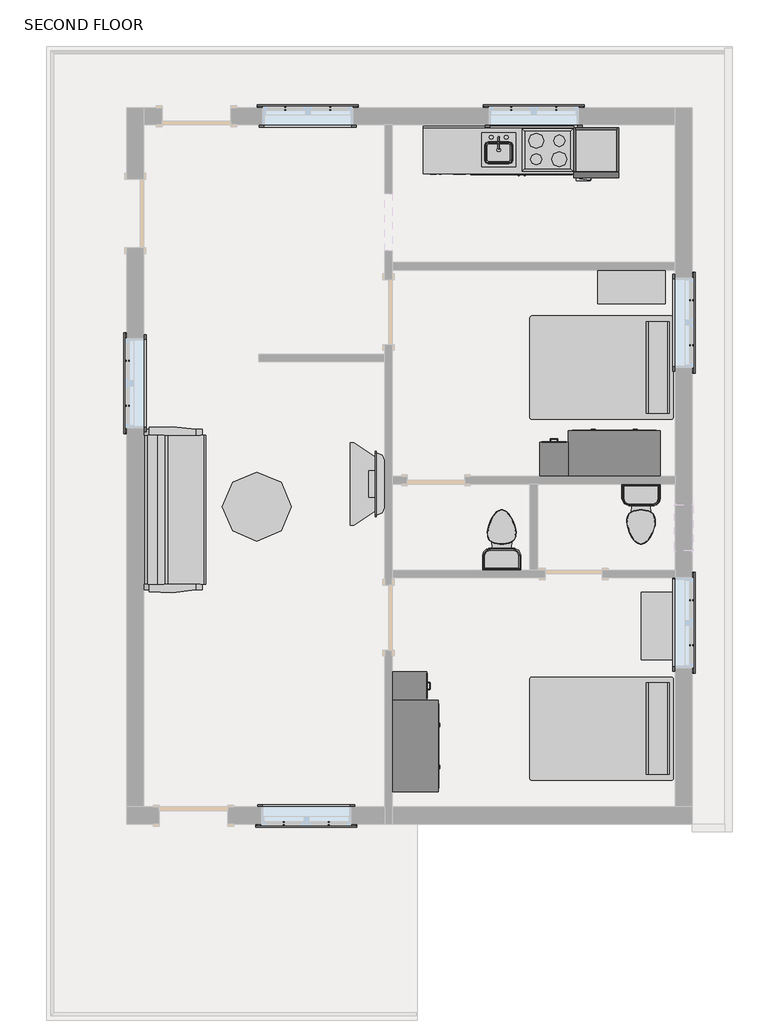
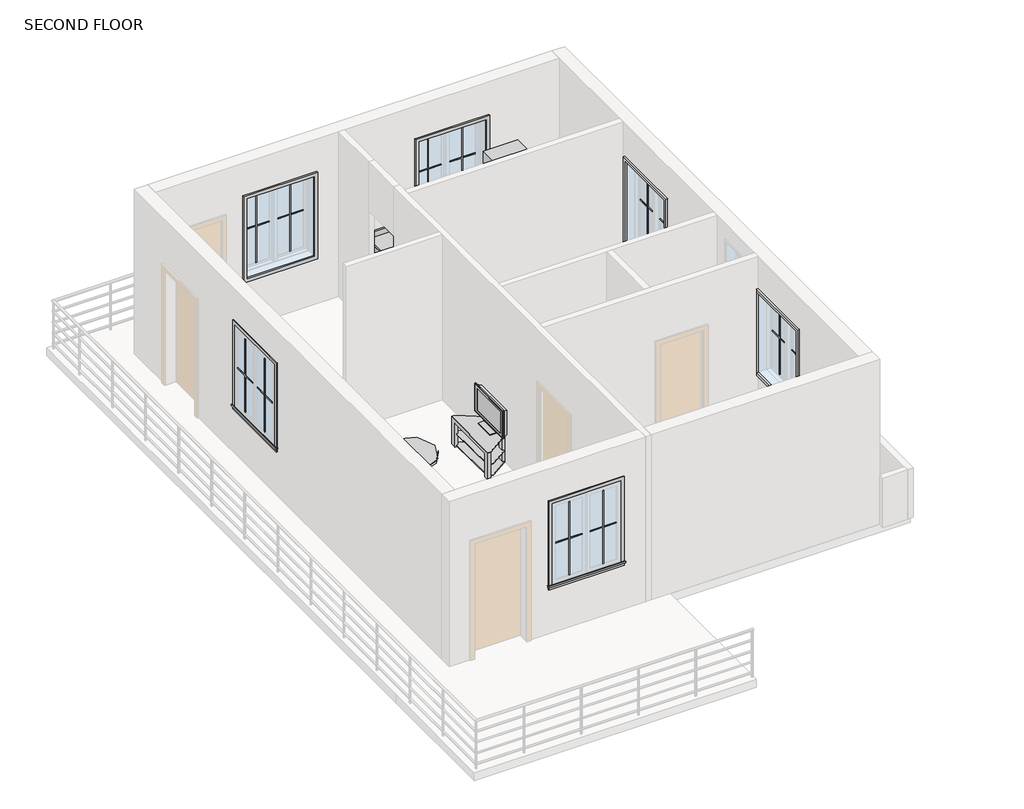
# One storey, part 3 of 3: 28 proxies, 13 furniture elements, 3 flow terminals.
"""IFC4 building model written with IfcOpenShell, lengths in millimetres."""

from ifc_helpers import new_model, si_unit, origin, place, context, project, spatial, transform, mapped, element, save
from components import m_cook_top_4_unit2_0615_x_500mm_c91639ce, m_dishwasher_610_x_610_x_875mm_75336c20, m_kitchenette_medium_m_kitchenette_medium_71e50c56, m_muntin_pattern_2x2_m_muntin_pattern_2x2_d4676b39, m_muntin_pattern_2x2_m_muntin_pattern_2x2_dce6eb8c, m_refrigerator_600_x_660mm_0a899b9c, m_trim_window_exterior_flat_with_sill_a970d7bf, m_trim_window_interior_flat_picture_frame_5bf35ee4, m_sink_kitchen_island_450_x_450mm_f6c2c534, m_toilet_domestic_3d_m_toilet_domestic_3d_ba6479b0, m_toilet_domestic_3d_m_toilet_domestic_3d_1a010dbe, furniture_dc210597, furniture_0810mm_51289c3c, m_bed_standard_1372_x_1905mm_double_64e02cd7, m_cabinet_file_5_drawer_0380_x_0457mm_21dee09a, m_counter_top_w_sink_hole_600mm_depth_2c7d9717, m_dresser_1220_x_1830_x_0610mm_75a9f440, m_furniture_system_storage_cabinet_2_vertical_file_900_x_450_def3fd80, m_sofa_pensi_2134mm_538a523a, m_table_dining_round_0915mm_diameter_394c0b6d

model = new_model("IFC4")

# Units and contexts
model_context = context("Model", 3, world=origin())
ifc_project = project(units=[si_unit("LENGTHUNIT", "METRE", prefix="MILLI")], contexts=[model_context])

# Site, building, storey
site = spatial("IfcSite", under=ifc_project)
building = spatial("IfcBuilding", under=site)
storey = spatial("IfcBuildingStorey", under=building, Name="SECOND FLOOR", Elevation=6400.8)

# Proxies
placement = place(None, origin())
m_cook_top_4_unit2_0615_x_500mm_shape = m_cook_top_4_unit2_0615_x_500mm_c91639ce(model_context)
element("IfcBuildingElementProxy", 1, Name="M_Cook Top-4 Unit2 : 0615 x 500mm", ObjectType="M_Cook Top-4 Unit2 : 0615 x 500mm", at=placement, inside=storey, context=model_context, shape_type="MappedRepresentation", body=[
    mapped(m_cook_top_4_unit2_0615_x_500mm_shape, transform((1952.0701854, 4546.4851347, 6415.8), x_axis=(-1.0, 0.0, 0.0), y_axis=(0.0, -1.0, 0.0), z_axis=(0.0, 0.0, 1.0))),
])
m_dishwasher_610_x_610_x_875mm_shape = m_dishwasher_610_x_610_x_875mm_75336c20(model_context)
element("IfcBuildingElementProxy", 2, Name="M_Dishwasher : 610 x 610 x 875mm", ObjectType="M_Dishwasher : 610 x 610 x 875mm", at=placement, inside=storey, context=model_context, shape_type="MappedRepresentation", body=[
    mapped(m_dishwasher_610_x_610_x_875mm_shape, transform((987.0876539, 4289.8355699, 6400.8), x_axis=(-1.0, 0.0, 0.0), y_axis=(0.0, -1.0, 0.0), z_axis=(0.0, 0.0, 1.0))),
])
m_kitchenette_medium_m_kitchenette_medium_shape = m_kitchenette_medium_m_kitchenette_medium_71e50c56(model_context)
element("IfcBuildingElementProxy", 3, Name="M_Kitchenette - Medium : M_Kitchenette - Medium", ObjectType="M_Kitchenette - Medium : M_Kitchenette - Medium", at=placement, inside=storey, context=model_context, shape_type="MappedRepresentation", body=[
    mapped(m_kitchenette_medium_m_kitchenette_medium_shape, transform((1623.3078903, 4861.4851347, 6400.8), x_axis=(-1.0, 0.0, 0.0), y_axis=(0.0, -1.0, 0.0), z_axis=(0.0, 0.0, 1.0))),
])
m_muntin_pattern_2x2_m_muntin_pattern_2x2_shape = m_muntin_pattern_2x2_m_muntin_pattern_2x2_d4676b39(model_context)
element("IfcBuildingElementProxy", 4, Name="M_Muntin Pattern_2x2 : M_Muntin Pattern_2x2", ObjectType="M_Muntin Pattern_2x2 : M_Muntin Pattern_2x2", at=placement, inside=storey, context=model_context, shape_type="MappedRepresentation", body=[
    mapped(m_muntin_pattern_2x2_m_muntin_pattern_2x2_shape, transform((1466.9330952, 5099.6101347, 7370.65), x_axis=(1.0, 0.0, 0.0), y_axis=(0.0, 1.0, 0.0), z_axis=(0.0, 0.0, 1.0))),
])
element("IfcBuildingElementProxy", 5, Name="M_Muntin Pattern_2x2 : M_Muntin Pattern_2x2", ObjectType="M_Muntin Pattern_2x2 : M_Muntin Pattern_2x2", at=placement, inside=storey, context=model_context, shape_type="MappedRepresentation", body=[
    mapped(m_muntin_pattern_2x2_m_muntin_pattern_2x2_shape, transform((3864.0205952, 2548.5476347, 7370.65), x_axis=(0.0, -1.0, 0.0), y_axis=(1.0, 0.0, 0.0), z_axis=(0.0, 0.0, 1.0))),
])
element("IfcBuildingElementProxy", 6, Name="M_Muntin Pattern_2x2 : M_Muntin Pattern_2x2", ObjectType="M_Muntin Pattern_2x2 : M_Muntin Pattern_2x2", at=placement, inside=storey, context=model_context, shape_type="MappedRepresentation", body=[
    mapped(m_muntin_pattern_2x2_m_muntin_pattern_2x2_shape, transform((3864.0205952, -1440.8523653, 7370.65), x_axis=(0.0, -1.0, 0.0), y_axis=(1.0, 0.0, 0.0), z_axis=(0.0, 0.0, 1.0))),
])
element("IfcBuildingElementProxy", 7, Name="M_Muntin Pattern_2x2 : M_Muntin Pattern_2x2", ObjectType="M_Muntin Pattern_2x2 : M_Muntin Pattern_2x2", at=placement, inside=storey, context=model_context, shape_type="MappedRepresentation", body=[
    mapped(m_muntin_pattern_2x2_m_muntin_pattern_2x2_shape, transform((-3635.3294048, 1147.1226347, 7370.65), x_axis=(0.0, 1.0, 0.0), y_axis=(-1.0, 0.0, 0.0), z_axis=(0.0, 0.0, 1.0))),
])
element("IfcBuildingElementProxy", 8, Name="M_Muntin Pattern_2x2 : M_Muntin Pattern_2x2", ObjectType="M_Muntin Pattern_2x2 : M_Muntin Pattern_2x2", at=placement, inside=storey, context=model_context, shape_type="MappedRepresentation", body=[
    mapped(m_muntin_pattern_2x2_m_muntin_pattern_2x2_shape, transform((-1536.9669048, 5099.6101347, 7370.65), x_axis=(1.0, 0.0, 0.0), y_axis=(0.0, 1.0, 0.0), z_axis=(0.0, 0.0, 1.0))),
])
element("IfcBuildingElementProxy", 9, Name="M_Muntin Pattern_2x2 : M_Muntin Pattern_2x2", ObjectType="M_Muntin Pattern_2x2 : M_Muntin Pattern_2x2", at=placement, inside=storey, context=model_context, shape_type="MappedRepresentation", body=[
    mapped(m_muntin_pattern_2x2_m_muntin_pattern_2x2_shape, transform((-960.1419048, -4406.3398653, 7370.65), x_axis=(-1.0, 0.0, 0.0), y_axis=(0.0, -1.0, 0.0), z_axis=(0.0, 0.0, 1.0))),
])
m_muntin_pattern_2x2_m_muntin_pattern_2x2_2_shape = m_muntin_pattern_2x2_m_muntin_pattern_2x2_dce6eb8c(model_context)
element("IfcBuildingElementProxy", 10, Name="M_Muntin Pattern_2x2 : M_Muntin Pattern_2x2", ObjectType="M_Muntin Pattern_2x2 : M_Muntin Pattern_2x2", at=placement, inside=storey, context=model_context, shape_type="MappedRepresentation", body=[
    mapped(m_muntin_pattern_2x2_m_muntin_pattern_2x2_2_shape, transform((2063.7580952, 5099.6101347, 7370.65), x_axis=(-1.0, 0.0, 0.0), y_axis=(0.0, -1.0, 0.0), z_axis=(0.0, 0.0, 1.0))),
])
element("IfcBuildingElementProxy", 11, Name="M_Muntin Pattern_2x2 : M_Muntin Pattern_2x2", ObjectType="M_Muntin Pattern_2x2 : M_Muntin Pattern_2x2", at=placement, inside=storey, context=model_context, shape_type="MappedRepresentation", body=[
    mapped(m_muntin_pattern_2x2_m_muntin_pattern_2x2_2_shape, transform((3864.0205952, 1951.7226347, 7370.65), x_axis=(0.0, 1.0, 0.0), y_axis=(-1.0, 0.0, 0.0), z_axis=(0.0, 0.0, 1.0))),
])
element("IfcBuildingElementProxy", 12, Name="M_Muntin Pattern_2x2 : M_Muntin Pattern_2x2", ObjectType="M_Muntin Pattern_2x2 : M_Muntin Pattern_2x2", at=placement, inside=storey, context=model_context, shape_type="MappedRepresentation", body=[
    mapped(m_muntin_pattern_2x2_m_muntin_pattern_2x2_2_shape, transform((3864.0205952, -2037.6773653, 7370.65), x_axis=(0.0, 1.0, 0.0), y_axis=(-1.0, 0.0, 0.0), z_axis=(0.0, 0.0, 1.0))),
])
element("IfcBuildingElementProxy", 13, Name="M_Muntin Pattern_2x2 : M_Muntin Pattern_2x2", ObjectType="M_Muntin Pattern_2x2 : M_Muntin Pattern_2x2", at=placement, inside=storey, context=model_context, shape_type="MappedRepresentation", body=[
    mapped(m_muntin_pattern_2x2_m_muntin_pattern_2x2_2_shape, transform((-3635.3294048, 1743.9476347, 7370.65), x_axis=(0.0, -1.0, 0.0), y_axis=(1.0, 0.0, 0.0), z_axis=(0.0, 0.0, 1.0))),
])
element("IfcBuildingElementProxy", 14, Name="M_Muntin Pattern_2x2 : M_Muntin Pattern_2x2", ObjectType="M_Muntin Pattern_2x2 : M_Muntin Pattern_2x2", at=placement, inside=storey, context=model_context, shape_type="MappedRepresentation", body=[
    mapped(m_muntin_pattern_2x2_m_muntin_pattern_2x2_2_shape, transform((-940.1419048, 5099.6101347, 7370.65), x_axis=(-1.0, 0.0, 0.0), y_axis=(0.0, -1.0, 0.0), z_axis=(0.0, 0.0, 1.0))),
])
element("IfcBuildingElementProxy", 15, Name="M_Muntin Pattern_2x2 : M_Muntin Pattern_2x2", ObjectType="M_Muntin Pattern_2x2 : M_Muntin Pattern_2x2", at=placement, inside=storey, context=model_context, shape_type="MappedRepresentation", body=[
    mapped(m_muntin_pattern_2x2_m_muntin_pattern_2x2_2_shape, transform((-1556.9669048, -4406.3398653, 7370.65), x_axis=(1.0, 0.0, 0.0), y_axis=(0.0, 1.0, 0.0), z_axis=(0.0, 0.0, 1.0))),
])
m_refrigerator_600_x_660mm_shape = m_refrigerator_600_x_660mm_0a899b9c(model_context)
element("IfcBuildingElementProxy", 16, Name="M_Refrigerator : 600 x 660mm", ObjectType="M_Refrigerator : 600 x 660mm", at=placement, inside=storey, context=model_context, shape_type="MappedRepresentation", body=[
    mapped(m_refrigerator_600_x_660mm_shape, transform((2541.7251841, 4544.3679413, 6400.8), x_axis=(-1.0, 0.0, 0.0), y_axis=(0.0, -1.0, 0.0), z_axis=(0.0, 0.0, 1.0))),
])
m_trim_window_exterior_flat_with_sill_shape = m_trim_window_exterior_flat_with_sill_a970d7bf(model_context)
element("IfcBuildingElementProxy", 17, Name="M_Trim-Window-Exterior-Flat : with Sill", ObjectType="M_Trim-Window-Exterior-Flat : with Sill", at=placement, inside=storey, context=model_context, shape_type="MappedRepresentation", body=[
    mapped(m_trim_window_exterior_flat_with_sill_shape, transform((1765.3455952, 5109.1351347, 8800.8), x_axis=(-1.0, 0.0, 0.0), y_axis=(0.0, 0.0, 1.0), z_axis=(0.0, 1.0, 0.0))),
])
element("IfcBuildingElementProxy", 18, Name="M_Trim-Window-Exterior-Flat : with Sill", ObjectType="M_Trim-Window-Exterior-Flat : with Sill", at=placement, inside=storey, context=model_context, shape_type="MappedRepresentation", body=[
    mapped(m_trim_window_exterior_flat_with_sill_shape, transform((3873.5455952, 2250.1351347, 8800.8), x_axis=(0.0, 1.0, 0.0), y_axis=(0.0, 0.0, 1.0), z_axis=(1.0, 0.0, 0.0))),
])
element("IfcBuildingElementProxy", 19, Name="M_Trim-Window-Exterior-Flat : with Sill", ObjectType="M_Trim-Window-Exterior-Flat : with Sill", at=placement, inside=storey, context=model_context, shape_type="MappedRepresentation", body=[
    mapped(m_trim_window_exterior_flat_with_sill_shape, transform((3873.5455952, -1739.2648653, 8800.8), x_axis=(0.0, 1.0, 0.0), y_axis=(0.0, 0.0, 1.0), z_axis=(1.0, 0.0, 0.0))),
])
element("IfcBuildingElementProxy", 20, Name="M_Trim-Window-Exterior-Flat : with Sill", ObjectType="M_Trim-Window-Exterior-Flat : with Sill", at=placement, inside=storey, context=model_context, shape_type="MappedRepresentation", body=[
    mapped(m_trim_window_exterior_flat_with_sill_shape, transform((-3644.8544048, 1445.5351347, 8800.8), x_axis=(0.0, -1.0, 0.0), y_axis=(0.0, 0.0, 1.0), z_axis=(-1.0, 0.0, 0.0))),
])
element("IfcBuildingElementProxy", 21, Name="M_Trim-Window-Exterior-Flat : with Sill", ObjectType="M_Trim-Window-Exterior-Flat : with Sill", at=placement, inside=storey, context=model_context, shape_type="MappedRepresentation", body=[
    mapped(m_trim_window_exterior_flat_with_sill_shape, transform((-1238.5544048, 5109.1351347, 8800.8), x_axis=(-1.0, 0.0, 0.0), y_axis=(0.0, 0.0, 1.0), z_axis=(0.0, 1.0, 0.0))),
])
element("IfcBuildingElementProxy", 22, Name="M_Trim-Window-Exterior-Flat : with Sill", ObjectType="M_Trim-Window-Exterior-Flat : with Sill", at=placement, inside=storey, context=model_context, shape_type="MappedRepresentation", body=[
    mapped(m_trim_window_exterior_flat_with_sill_shape, transform((-1258.5544048, -4415.8648653, 8800.8), x_axis=(1.0, 0.0, 0.0), y_axis=(0.0, 0.0, 1.0), z_axis=(0.0, -1.0, 0.0))),
])
m_trim_window_interior_flat_picture_frame_shape = m_trim_window_interior_flat_picture_frame_5bf35ee4(model_context)
element("IfcBuildingElementProxy", 23, Name="M_Trim-Window-Interior-Flat : Picture Frame", ObjectType="M_Trim-Window-Interior-Flat : Picture Frame", at=placement, inside=storey, context=model_context, shape_type="MappedRepresentation", body=[
    mapped(m_trim_window_interior_flat_picture_frame_shape, transform((1765.3455952, 4880.5351347, 8800.8), x_axis=(1.0, 0.0, 0.0), y_axis=(0.0, 0.0, 1.0), z_axis=(0.0, -1.0, 0.0))),
])
element("IfcBuildingElementProxy", 24, Name="M_Trim-Window-Interior-Flat : Picture Frame", ObjectType="M_Trim-Window-Interior-Flat : Picture Frame", at=placement, inside=storey, context=model_context, shape_type="MappedRepresentation", body=[
    mapped(m_trim_window_interior_flat_picture_frame_shape, transform((3644.9455952, 2250.1351347, 8800.8), x_axis=(0.0, -1.0, 0.0), y_axis=(0.0, 0.0, 1.0), z_axis=(-1.0, 0.0, 0.0))),
])
element("IfcBuildingElementProxy", 25, Name="M_Trim-Window-Interior-Flat : Picture Frame", ObjectType="M_Trim-Window-Interior-Flat : Picture Frame", at=placement, inside=storey, context=model_context, shape_type="MappedRepresentation", body=[
    mapped(m_trim_window_interior_flat_picture_frame_shape, transform((3644.9455952, -1739.2648653, 8800.8), x_axis=(0.0, -1.0, 0.0), y_axis=(0.0, 0.0, 1.0), z_axis=(-1.0, 0.0, 0.0))),
])
element("IfcBuildingElementProxy", 26, Name="M_Trim-Window-Interior-Flat : Picture Frame", ObjectType="M_Trim-Window-Interior-Flat : Picture Frame", at=placement, inside=storey, context=model_context, shape_type="MappedRepresentation", body=[
    mapped(m_trim_window_interior_flat_picture_frame_shape, transform((-3416.2544048, 1445.5351347, 8800.8), x_axis=(0.0, 1.0, 0.0), y_axis=(0.0, 0.0, 1.0), z_axis=(1.0, 0.0, 0.0))),
])
element("IfcBuildingElementProxy", 27, Name="M_Trim-Window-Interior-Flat : Picture Frame", ObjectType="M_Trim-Window-Interior-Flat : Picture Frame", at=placement, inside=storey, context=model_context, shape_type="MappedRepresentation", body=[
    mapped(m_trim_window_interior_flat_picture_frame_shape, transform((-1238.5544048, 4880.5351347, 8800.8), x_axis=(1.0, 0.0, 0.0), y_axis=(0.0, 0.0, 1.0), z_axis=(0.0, -1.0, 0.0))),
])
element("IfcBuildingElementProxy", 28, Name="M_Trim-Window-Interior-Flat : Picture Frame", ObjectType="M_Trim-Window-Interior-Flat : Picture Frame", at=placement, inside=storey, context=model_context, shape_type="MappedRepresentation", body=[
    mapped(m_trim_window_interior_flat_picture_frame_shape, transform((-1258.5544048, -4187.2648653, 8800.8), x_axis=(-1.0, 0.0, 0.0), y_axis=(0.0, 0.0, 1.0), z_axis=(0.0, 1.0, 0.0))),
])

# Flow terminals
m_sink_kitchen_island_450_x_450mm_shape = m_sink_kitchen_island_450_x_450mm_f6c2c534(model_context)
element("IfcFlowTerminal", 29, ObjectType="M_Sink Kitchen-Island : 450 x 450mm", at=placement, inside=storey, context=model_context, shape_type="MappedRepresentation", body=[
    mapped(m_sink_kitchen_island_450_x_450mm_shape, transform((1315.2594259, 4546.0397336, 6415.8), x_axis=(-1.0, 0.0, 0.0), y_axis=(0.0, -1.0, 0.0), z_axis=(0.0, 0.0, 1.0))),
])
m_toilet_domestic_3d_m_toilet_domestic_3d_shape = m_toilet_domestic_3d_m_toilet_domestic_3d_ba6479b0(model_context)
m_toilet_domestic_3d_m_toilet_domestic_3d_2_shape = m_toilet_domestic_3d_m_toilet_domestic_3d_1a010dbe(model_context)
element("IfcFlowTerminal", 30, ObjectType="M_Toilet-Domestic-3D : M_Toilet-Domestic-3D", at=placement, inside=storey, context=model_context, shape_type="MappedRepresentation", body=[
    mapped(m_toilet_domestic_3d_m_toilet_domestic_3d_shape, transform((3191.5495678, -389.3608926, 6400.8), x_axis=(1.0, 0.0, 0.0), y_axis=(0.0, 1.0, 0.0), z_axis=(0.0, 0.0, 1.0))),
    mapped(m_toilet_domestic_3d_m_toilet_domestic_3d_2_shape, transform((3191.5495678, -389.3608926, 6400.8), x_axis=(1.0, 0.0, 0.0), y_axis=(0.0, 1.0, 0.0), z_axis=(0.0, 0.0, 1.0))),
])
element("IfcFlowTerminal", 31, ObjectType="M_Toilet-Domestic-3D : M_Toilet-Domestic-3D", at=placement, inside=storey, context=model_context, shape_type="MappedRepresentation", body=[
    mapped(m_toilet_domestic_3d_m_toilet_domestic_3d_shape, transform((1339.1416225, -542.9688379, 6400.8), x_axis=(-1.0, 0.0, 0.0), y_axis=(0.0, -1.0, 0.0), z_axis=(0.0, 0.0, 1.0))),
    mapped(m_toilet_domestic_3d_m_toilet_domestic_3d_2_shape, transform((1339.1416225, -542.9688379, 6400.8), x_axis=(-1.0, 0.0, 0.0), y_axis=(0.0, -1.0, 0.0), z_axis=(0.0, 0.0, 1.0))),
])

# Furniture
furniture_shape = furniture_dc210597(model_context)
element("IfcFurniture", 32, at=placement, inside=storey, context=model_context, shape_type="MappedRepresentation", body=[
    mapped(furniture_shape, transform((-215.8544048, 230.5231368, 6400.8), x_axis=(0.0, -1.0, 0.0), y_axis=(1.0, 0.0, 0.0), z_axis=(0.0, 0.0, 1.0))),
])
furniture_0810mm_shape = furniture_0810mm_51289c3c(model_context)
element("IfcFurniture", 33, ObjectType="0810mm", at=placement, inside=storey, context=model_context, shape_type="MappedRepresentation", body=[
    mapped(furniture_0810mm_shape, transform((-274.3930285, 101.3906206, 6910.8), x_axis=(0.0, -1.0, 0.0), y_axis=(1.0, 0.0, 0.0), z_axis=(0.0, 0.0, 1.0))),
])
m_bed_standard_1372_x_1905mm_double_shape = m_bed_standard_1372_x_1905mm_double_64e02cd7(model_context)
element("IfcFurniture", 34, ObjectType="M_Bed-Standard : 1372 x 1905mm - Double", at=placement, inside=storey, context=model_context, shape_type="MappedRepresentation", body=[
    mapped(m_bed_standard_1372_x_1905mm_double_shape, transform((2712.6406772, -2874.5763407, 6400.8), x_axis=(0.0, -1.0, 0.0), y_axis=(1.0, 0.0, 0.0), z_axis=(0.0, 0.0, 1.0))),
])
element("IfcFurniture", 35, ObjectType="M_Bed-Standard : 1372 x 1905mm - Double", at=placement, inside=storey, context=model_context, shape_type="MappedRepresentation", body=[
    mapped(m_bed_standard_1372_x_1905mm_double_shape, transform((2712.6406772, 1925.4236593, 6400.8), x_axis=(0.0, -1.0, 0.0), y_axis=(1.0, 0.0, 0.0), z_axis=(0.0, 0.0, 1.0))),
])
m_cabinet_file_5_drawer_0380_x_0457mm_shape = m_cabinet_file_5_drawer_0380_x_0457mm_21dee09a(model_context)
element("IfcFurniture", 36, ObjectType="M_Cabinet-File 5 Drawer : 0380 x 0457mm", at=placement, inside=storey, context=model_context, shape_type="MappedRepresentation", body=[
    mapped(m_cabinet_file_5_drawer_0380_x_0457mm_shape, transform((-27.8887049, -2449.3684182, 6400.8), x_axis=(0.0, 1.0, 0.0), y_axis=(-1.0, 0.0, 0.0), z_axis=(0.0, 0.0, 1.0))),
])
element("IfcFurniture", 37, ObjectType="M_Cabinet-File 5 Drawer : 0380 x 0457mm", at=placement, inside=storey, context=model_context, shape_type="MappedRepresentation", body=[
    mapped(m_cabinet_file_5_drawer_0380_x_0457mm_shape, transform((1907.0491482, 293.3008346, 6400.8), x_axis=(-1.0, 0.0, 0.0), y_axis=(0.0, -1.0, 0.0), z_axis=(0.0, 0.0, 1.0))),
])
m_counter_top_w_sink_hole_600mm_depth_shape = m_counter_top_w_sink_hole_600mm_depth_2c7d9717(model_context)
element("IfcFurniture", 38, ObjectType="M_Counter Top w Sink Hole : 600mm Depth", at=placement, inside=storey, context=model_context, shape_type="MappedRepresentation", body=[
    mapped(m_counter_top_w_sink_hole_600mm_depth_shape, transform((1099.1078903, 4861.4851347, 6415.8), x_axis=(-1.0, 0.0, 0.0), y_axis=(0.0, -1.0, 0.0), z_axis=(0.0, 0.0, 1.0))),
])
m_dresser_1220_x_1830_x_0610mm_shape = m_dresser_1220_x_1830_x_0610mm_75a9f440(model_context)
element("IfcFurniture", 39, ObjectType="M_Dresser : 1220 x 1830 x 0610mm", at=placement, inside=storey, context=model_context, shape_type="MappedRepresentation", body=[
    mapped(m_dresser_1220_x_1830_x_0610mm_shape, transform((2565.7523354, 148.7721806, 6400.8), x_axis=(-1.0, 0.0, 0.0), y_axis=(0.0, -1.0, 0.0), z_axis=(0.0, 0.0, 1.0))),
])
element("IfcFurniture", 40, ObjectType="M_Dresser : 1220 x 1830 x 0610mm", at=placement, inside=storey, context=model_context, shape_type="MappedRepresentation", body=[
    mapped(m_dresser_1220_x_1830_x_0610mm_shape, transform((-172.4173589, -3108.0716054, 6400.8), x_axis=(0.0, 1.0, 0.0), y_axis=(-1.0, 0.0, 0.0), z_axis=(0.0, 0.0, 1.0))),
])
m_furniture_system_storage_cabinet_2_vertical_file_900_x_450_shape = m_furniture_system_storage_cabinet_2_vertical_file_900_x_450_def3fd80(model_context)
element("IfcFurniture", 41, ObjectType="M_Furniture_System-Storage-Cabinet-2_Vertical_File : 900 x 450 x 650mm", at=placement, inside=storey, context=model_context, shape_type="MappedRepresentation", body=[
    mapped(m_furniture_system_storage_cabinet_2_vertical_file_900_x_450_shape, transform((3066.1455952, 2500.1351347, 6400.8), x_axis=(1.0, 0.0, 0.0), y_axis=(0.0, 1.0, 0.0), z_axis=(0.0, 0.0, 1.0))),
])
element("IfcFurniture", 42, ObjectType="M_Furniture_System-Storage-Cabinet-2_Vertical_File : 900 x 450 x 650mm", at=placement, inside=storey, context=model_context, shape_type="MappedRepresentation", body=[
    mapped(m_furniture_system_storage_cabinet_2_vertical_file_900_x_450_shape, transform((3194.9455952, -1781.4648653, 6400.8), x_axis=(0.0, -1.0, 0.0), y_axis=(1.0, 0.0, 0.0), z_axis=(0.0, 0.0, 1.0))),
])
m_sofa_pensi_2134mm_shape = m_sofa_pensi_2134mm_538a523a(model_context)
element("IfcFurniture", 43, ObjectType="M_Sofa-Pensi : 2134mm", at=placement, inside=storey, context=model_context, shape_type="MappedRepresentation", body=[
    mapped(m_sofa_pensi_2134mm_shape, transform((-2738.7445687, -514.3711153, 6400.8), x_axis=(0.0, 1.0, 0.0), y_axis=(-1.0, 0.0, 0.0), z_axis=(0.0, 0.0, 1.0))),
])
m_table_dining_round_0915mm_diameter_shape = m_table_dining_round_0915mm_diameter_394c0b6d(model_context)
element("IfcFurniture", 44, ObjectType="M_Table-Dining Round : 0915mm Diameter", at=placement, inside=storey, context=model_context, shape_type="MappedRepresentation", body=[
    mapped(m_table_dining_round_0915mm_diameter_shape, transform((-2019.536372, -9.7861767, 6400.8), x_axis=(1.0, 0.0, 0.0), y_axis=(0.0, 1.0, 0.0), z_axis=(0.0, 0.0, 1.0))),
])

save(model, "model.ifc")

# Revit data of these elements
# Type "M_Cook Top-4 Unit2 : 0615 x 500mm"
#   Depth = 1.64042 ft
#   Width = 2.017717 ft
#   Burner Material = Steel, Chrome Plated
#   Cooktop Material = Steel, Polished
#   Default Elevation = 0
#   Assembly Code = ""
# Type "M_Dishwasher : 610 x 610 x 875mm"
#   Label = "DW"
#   Depth = 2.001312 ft
#   Height = 2.870735 ft
#   Width = 2.001312 ft
#   Dishwasher Material = Steel, Paint Finish, Ivory, Glossy
#   Panel Face Material = Plastic, Opaque Black
#   Default Elevation = 0
# Type "M_Kitchenette - Medium : M_Kitchenette - Medium"
#   Sink Opening Depth = 1.148294 ft
#   Sink Location To Wall = 0.492126 ft
#   Sink Location = 3.28084 ft
#   Counter Thickness = 0.131234 ft
#   Counter Length = 6.56168 ft
#   Cabinet Width = 4.560367 ft
#   Cabinet Height = 2.870735 ft
#   Cabinet Depth = 2.066929 ft
#   Toe Depth = 0.114829 ft
#   Toe Height = 0.328084 ft
#   Cabinet Material = Cabinets
#   Door/Drawer Material = Cabinets
#   Handle Material = Cabinets - Handles
#   Default Elevation = 0
# Type "M_Muntin Pattern_2x2 : M_Muntin Pattern_2x2"
#   Width [instance default] = 3.937008 ft
#   Thickness = 0.041667 ft
#   Height [instance default] = 3.937008 ft
#   Distance = 0.0625 ft
#   Interior Material [instance default] = none
#   Exterior Material [instance default] = none
#   Default Elevation = 0
# Type "M_Refrigerator : 600 x 660mm"
#   Label = "REF."
#   Depth = 2.165354 ft
#   Height = 6.003937 ft
#   Width = 1.968504 ft
#   Material = Steel, Paint Finish, Ivory, Matte
#   Description = (empty or 0)
#   Default Elevation = 0
# Type "M_Trim-Window-Exterior-Flat : with Sill"
#   Trim Width = 0.19685 ft
#   Trim Thickness_Picture Frame = 0.098425 ft
#   Trim Thickness_with Sill = 0.0625 ft
#   Sill Thickness = 0.098425 ft
#   Opening Width [instance default] = 1.968504 ft
#   Opening Height [instance default] = 2.952756 ft
#   Default Elevation = 3.937008 ft
#   Sill = yes
#   Picture Frame = no
#   Trim Material [instance default] = none
# Type "M_Trim-Window-Interior-Flat : Picture Frame"
#   Trim Thickness_Picture Frame = 0.098425 ft
#   Trim Width = 0.19685 ft
#   Trim Thickness_with Sill = 0.065617 ft
#   Sill Thickness = 0.098425 ft
#   Opening Width [instance default] = 1.968504 ft
#   Opening Height [instance default] = 2.952756 ft
#   Default Elevation = 3.937008 ft
#   Sill = no
#   Picture Frame = yes
#   Trim Material [instance default] = none
# Type "M_Sink Kitchen-Island : 450 x 450mm"
#   Counter Height [instance default] = 2.952756 ft
#   Depth = 1.476378 ft
#   Width = 1.476378 ft
#   Fixture Material = Steel, Polished
#   Sink Material = Steel, Polished
#   Default Elevation = 0
# Type "M_Toilet-Domestic-3D : M_Toilet-Domestic-3D"
#   Bowl/Basin Material = Porcelain, Linen
#   Seat Material = Laminate, Linen, Matte
#   Default Elevation = 0
# Type
#   Depth = 1.509186 ft
#   Width = 3.608924 ft
#   Height = 1.64042 ft
#   Finish = Melamine - Gray
#   Default Elevation = 0
# Type "0810mm"
#   SinAng = 0.001609 ft
#   L = 2.316144 ft
#   H = 1.30295 ft
#   Thickness = 0.360892 ft
#   Diagonal = 2.65748 ft
#   CosAng = 0.002859 ft
#   Stand [instance default] = yes
#   Default Elevation = 0
# Type "M_Bed-Standard : 1372 x 1905mm - Double"
#   Length = 6.25 ft
#   Width = 4.501312 ft
#   Leg Material = Steel, Chrome Plated
#   Mattress Material = Linen, White
#   Default Elevation = 0
# Type "M_Cabinet-File 5 Drawer : 0380 x 0457mm"
#   Depth = 1.499344 ft
#   Height = 5.003281 ft
#   Width = 1.246719 ft
#   Cabinet Material = Steel, Paint Finish, Ivory, Glossy
#   Handle Material = Steel, Chrome Plated
#   Default Elevation = 0
# Type "M_Counter Top w Sink Hole : 600mm Depth"
#   Counter Thickness = 0.131234 ft
#   Depth [instance default] = 2.050525 ft
#   Height = 2.952756 ft
#   Length [instance default] = 8.2021 ft
#   Sink Location [instance default] = 3.937008 ft
#   Sink Location To Wall [instance default] = 0.328084 ft
#   Sink Opening Depth [instance default] = 1.240157 ft
#   Sink Opening Width [instance default] = 1.925853 ft
#   Counter Top Material = none
#   Default Elevation = 0
# Type "M_Dresser : 1220 x 1830 x 0610mm"
#   Depth = 2.001312 ft
#   Height = 6.003937 ft
#   Width = 4.002625 ft
#   Dresser Material = Laminate - Ivory, Glossy
#   Drawer Material = Laminate, Ivory, Matte
#   Knob Material = Cherry
#   Default Elevation = 0
# Type "M_Furniture_System-Storage-Cabinet-2_Vertical_File : 900 x 450 x 650mm"
#   Type Comments = "900 x 450 x 650mm Double Vertical File Cabinet"
#   Width = 2.952756 ft
#   Height = 2.132546 ft
#   Depth = 1.476378 ft
#   Show Solid [instance default] = yes
#   Show Dashed [instance default] = no
#   Drawer Finish [instance default] = Metal - Paint - Beige
#   Cabinet Material [instance default] = Metal - Paint - Beige
#   Model = ""
#   Manufacturer = ""
#   Description = (empty or 0)
#   Default Elevation = 0
# Type "M_Sofa-Pensi : 2134mm"
#   Length = 7.001312 ft
#   Sofa Material = Linen, Beige
#   Frame Material = Steel, Chrome Plated
#   Default Elevation = 0
# Type "M_Table-Dining Round : 0915mm Diameter"
#   Diameter = 3.001969 ft
#   Height = 2.5 ft
#   Base Material = Pine
#   Top Material = Laminate, Linen, Matte
#   Default Elevation = 0
# Element 1 (IfcBuildingElementProxy, "M_Cook Top-4 Unit2 : 0615 x 500mm")
#   Phase Created = New Construction
#   Materials on its faces: "Steel, Polished", "Steel, Chrome Plated"
# Element 2 (IfcBuildingElementProxy, "M_Dishwasher : 610 x 610 x 875mm")
#   Phase Created = New Construction
#   Materials on its faces: "Steel, Paint Finish, Ivory, Glossy", "Plastic, Opaque Black"
# Element 3 (IfcBuildingElementProxy, "M_Kitchenette - Medium : M_Kitchenette - Medium")
#   Phase Created = New Construction
#   Materials on its faces: "Cabinets", "Cabinets - Handles"
# Elements 4, 5, 6, 7, 8, 9, 10, 11, 12, 13, 14, 15 (IfcBuildingElementProxy, "M_Muntin Pattern_2x2 : M_Muntin Pattern_2x2")
#   Width = 1.520587 ft
#   Height = 4.462927 ft
#   Interior Material = Wood - Stained
#   Exterior Material = Clad - White
#   Phase Created = New Construction
#   Materials on its faces: "Clad - White", "Wood - Stained"
# Element 16 (IfcBuildingElementProxy, "M_Refrigerator : 600 x 660mm")
#   Phase Created = New Construction
#   Materials on its faces: "Steel, Paint Finish, Ivory, Matte", "Steel, Chrome Plated"
# Elements 17, 18, 19, 20, 21, 22 (IfcBuildingElementProxy, "M_Trim-Window-Exterior-Flat : with Sill")
#   Opening Width = 3.937008 ft
#   Opening Height = 4.92126 ft
#   Trim Material = Clad - White
#   Phase Created = New Construction
#   Materials on its faces: "Clad - White"
# Elements 23, 24, 25, 26, 27, 28 (IfcBuildingElementProxy, "M_Trim-Window-Interior-Flat : Picture Frame")
#   Opening Width = 3.937008 ft
#   Opening Height = 4.92126 ft
#   Trim Material = Wood - Stained
#   Phase Created = New Construction
#   Materials on its faces: "Wood - Stained"
# Element 29 (IfcFlowTerminal, "M_Sink Kitchen-Island : 450 x 450mm")
#   Mark = "11"
#   Counter Height = 2.952756 ft
#   Phase Created = New Construction
#   Materials on its faces: "Steel, Polished"
# Element 30 (IfcFlowTerminal, "M_Toilet-Domestic-3D : M_Toilet-Domestic-3D")
#   Mark = "12"
#   Phase Created = New Construction
#   Materials on its faces: "Porcelain, Linen", "Laminate, Linen, Matte"
# Element 31 (IfcFlowTerminal, "M_Toilet-Domestic-3D : M_Toilet-Domestic-3D")
#   Mark = "13"
#   Phase Created = New Construction
#   Materials on its faces: "Porcelain, Linen", "Laminate, Linen, Matte"
# Element 32 (IfcFurniture)
#   Phase Created = New Construction
#   Materials on its faces: "Melamine - Gray", "Glass - Shelves"
# Element 33 (IfcFurniture, "0810mm")
#   Stand = yes
#   Phase Created = New Construction
#   Materials on its faces: "TV - Black", "TV - Glass", "TV - Screen"
# Elements 34, 35 (IfcFurniture, "M_Bed-Standard : 1372 x 1905mm - Double")
#   Phase Created = New Construction
#   Materials on its faces: "Linen, White", "Steel, Chrome Plated"
# Elements 36, 37 (IfcFurniture, "M_Cabinet-File 5 Drawer : 0380 x 0457mm")
#   Phase Created = New Construction
#   Materials on its faces: "Steel, Chrome Plated", "Steel, Paint Finish, Ivory, Glossy"
# Element 38 (IfcFurniture, "M_Counter Top w Sink Hole : 600mm Depth")
#   Sink Opening Width = 1.312336 ft
#   Sink Opening Depth = 1.148294 ft
#   Sink Location To Wall = 0.492126 ft
#   Sink Location = 3.28084 ft
#   Length = 6.56168 ft
#   Depth = 2.066929 ft
#   Phase Created = New Construction
#   Materials on its faces: "Counter Top"
# Elements 39, 40 (IfcFurniture, "M_Dresser : 1220 x 1830 x 0610mm")
#   Phase Created = New Construction
#   Materials on its faces: "Laminate, Ivory, Matte", "Cherry", "Laminate - Ivory, Glossy"
# Elements 41, 42 (IfcFurniture, "M_Furniture_System-Storage-Cabinet-2_Vertical_File : 900 x 450 x 650mm")
#   Show Solid = yes
#   Show Dashed = no
#   Drawer Finish = Metal - Paint - Beige
#   Cabinet Material = Metal - Paint - Beige
#   Phase Created = New Construction
#   Materials on its faces: "Metal - Paint - Beige"
# Element 43 (IfcFurniture, "M_Sofa-Pensi : 2134mm")
#   Phase Created = New Construction
#   Materials on its faces: "Linen, Beige", "Steel, Chrome Plated"
# Element 44 (IfcFurniture, "M_Table-Dining Round : 0915mm Diameter")
#   Phase Created = New Construction
#   Materials on its faces: "Pine", "Laminate, Linen, Matte"
# Materials
#   "Steel, Chrome Plated": class "Metal", colour RGB 17 17 17, transparency 0, Description = "Chromiuim plated steel", Cost = 0
#   "Steel, Polished": class "Metal", colour RGB 57 57 57, transparency 0, Description = "Polished steel", Cost = 0
#   "Steel, Paint Finish, Ivory, Glossy": class "Metal", colour RGB 247 247 239, transparency 0, Description = "Steel, paint finish, ivory, glossy", Cost = 0
#   "Plastic, Opaque Black": class "Plastic", colour RGB 0 0 0, transparency 0.7, Description = "Plastic, generic, opaque black", Cost = 0
#   "Cabinets": colour RGB 249 249 249, transparency 0
#   "Cabinets - Handles": class "Metal", colour RGB 57 57 57, transparency 0
#   "Steel, Paint Finish, Ivory, Matte": class "Metal", colour RGB 247 247 239, transparency 0, Description = "Steel, paint finish, ivory, matte", Cost = 0
#   "Porcelain, Linen": class "Ceramic", colour RGB 249 239 230, transparency 0, Description = "Porcelain, linen", Cost = 0
#   "Laminate, Linen, Matte": class "Plastic", colour RGB 249 239 230, transparency 0, Description = "Plastic Laminate - Linen, Matte", Cost = 0
#   "Melamine - Gray": class "Wood", colour RGB 49 49 49, transparency 0
#   "Linen, White": class "Textile", colour RGB 247 247 239, transparency 0, Description = "Linen, white", Cost = 0
#   "Laminate - Ivory, Glossy": colour RGB 247 247 239, transparency 0
#   "Laminate, Ivory, Matte": class "Plastic", colour RGB 247 247 239, transparency 0, Description = "Plastic Laminate - Ivory, Matte", Cost = 0
#   "Cherry": class "Wood", colour RGB 226 177 128, transparency 0, Description = "Prunus Serotina", Cost = 0
#   "Metal - Paint - Beige": class "Metal", colour RGB 247 225 182, transparency 0
#   "Linen, Beige": class "Textile", colour RGB 249 239 230, transparency 0, Description = "Linen, beige", Cost = 0
#   "Pine": class "Wood", colour RGB 223 192 134, transparency 0, Description = "Pinus Echinata", Cost = 0
#   "Clad - White": class "Wood", colour RGB 242 242 238, transparency 0, Cost = 0
#   "Wood - Stained": class "Wood", colour RGB 224 178 126, transparency 0, Cost = 0
#   "Glass - Shelves": class "Glass", colour RGB 167 167 167, transparency 0.9
#   "TV - Black": colour RGB 49 49 49, transparency 0
#   "TV - Glass": colour RGB 157 157 157, transparency 0.9
#   "TV - Screen": colour RGB 0 0 0, transparency 0
#   "Counter Top": class "Wood", colour RGB 226 177 128, transparency 0
